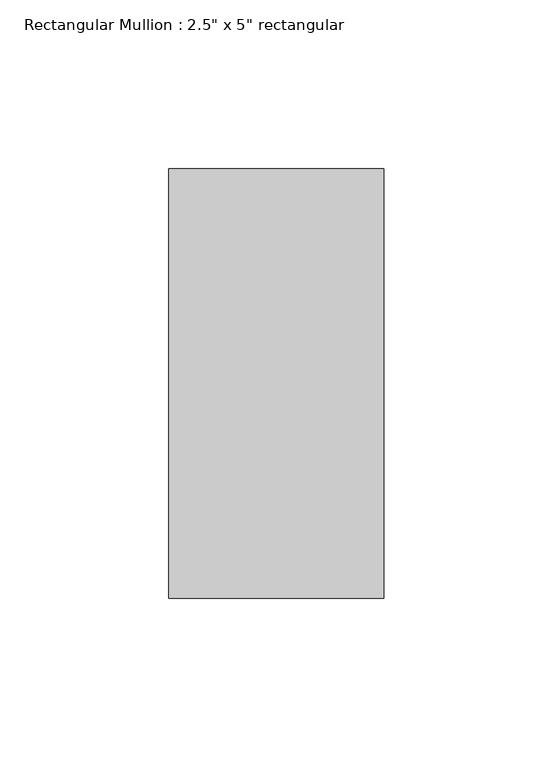
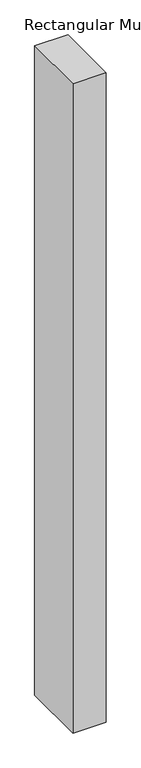
"""IFC4 building model written with IfcOpenShell, lengths in millimetres: member geometry."""

from ifc_helpers import new_model, si_unit, frame, origin, place, context, project, spatial, polyline, outline, extrude, source, transform, mapped, element, save


def member_b98e8178(model_context):
    return source(origin(), model_context, "Body", "SweptSolid", [
        extrude(outline(polyline([(0.0, 63.5), (0.0, -63.5), (-63.5, -63.5), (-63.5, 63.5), (0.0, 63.5)])), frame((0.0, 0.0, -1315.425758), z_axis=(0.0, 0.0, 1.0), x_axis=(1.0, 0.0, 0.0)), (0.0, 0.0, 1.0), 1315.425758),
    ])


if __name__ == "__main__":
    model = new_model("IFC4")
    model_context = context("Model", 3, world=origin())
    ifc_project = project(units=[si_unit("LENGTHUNIT", "METRE", prefix="MILLI")], contexts=[model_context])
    site = spatial("IfcSite", under=ifc_project)
    building = spatial("IfcBuilding", under=site)
    placement = place(None, origin())
    member_shape = member_b98e8178(model_context)
    element("IfcMember", 1, ObjectType="Rectangular Mullion : 2.5\" x 5\" rectangular", at=placement, inside=building, context=model_context, shape_type="MappedRepresentation", body=[
        mapped(member_shape, transform((0.0, 0.0, 0.0), x_axis=(1.0, 0.0, 0.0), y_axis=(0.0, 1.0, 0.0), z_axis=(0.0, 0.0, 1.0))),
    ])
    save(model, "model.ifc")

# Revit data of these elements
# Type "Rectangular Mullion : 2.5\" x 5\" rectangular"
#   built-in parameter 1007304 = 0.416667 (stored number, unit not read)
#   built-in parameter 1007301 = 0.104167 (stored number, unit not read)
#   built-in parameter 1007300 = 0.104167 (stored number, unit not read)
# Element 1 (IfcMember, "Rectangular Mullion : 2.5\" x 5\" rectangular")
#   Materials on its faces: "Aluminum"
# Materials
#   "Aluminum": class "Metal", colour RGB 247 247 247, transparency 0, Description = "Aluminum 6061", Cost = 0
